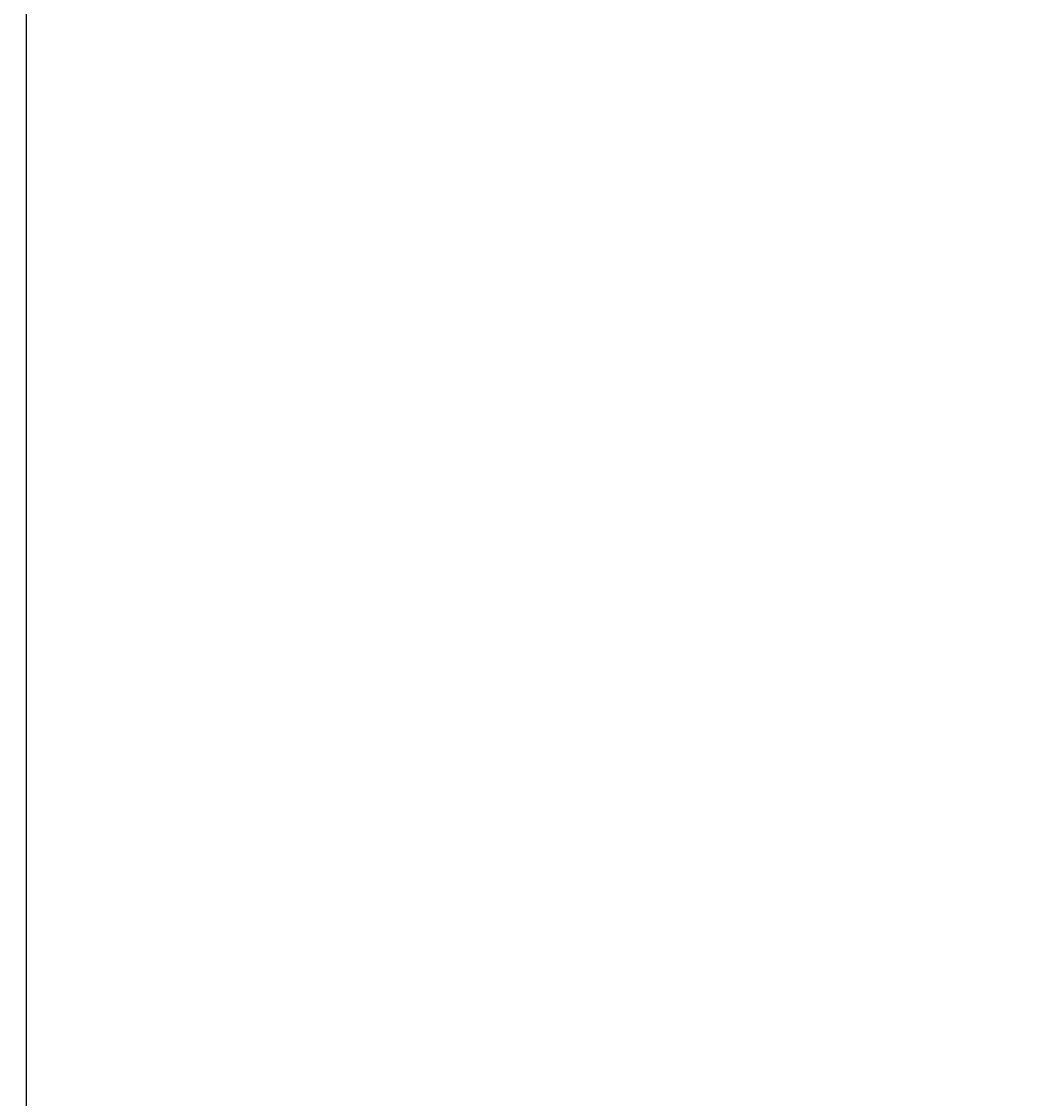
# Model space of a CAD drawing. Units: millimetres. Extents: x 27017497 to 27018854, y 7058029 to 7059154.
# Tile 2 of 91: x 27017497 to 27017560, y 7058133 to 7058200. Entities that reach past the tile are written whole.
import ezdxf

# ---------------------------------------------------------------- set-up
doc = ezdxf.new("R2010")
doc.units = ezdxf.units.MM
doc.layers.add('A-ANNO-DIMS', color=2, linetype='Continuous', lineweight=18)
doc.styles.get("Standard").update_dxf_attribs({"font": 'arial.ttf'})
doc.dimstyles.get("Standard").update_dxf_attribs({"dimtxt": 0.18, "dimasz": 0.18, "dimexe": 0.18, "dimexo": 0.0625, "dimgap": 0.09, "dimtad": 0, "dimtih": 1, "dimtoh": 1, "dimdec": 4, "dimzin": 0, "dimdsep": 46, "dimtxsty": 'Standard', "dimcen": 0.09, "dimadec": 0, "dimazin": 0, "dimtfac": 1, "dimtdec": 4, "dimtofl": 0, "dimtmove": 0, "dimatfit": 3, "dimfxl": 1, "dimtolj": 1, "dimtzin": 0, "dimarcsym": 0})

# ---------------------------------------------------------------- blocks, each defined once
blk = doc.blocks.new('*D48')
at = {"layer": 'A-ANNO-DIMS', "color": 0, "lineweight": -2, "transparency": 16777216}
for p, q in [((27018463.498, 7058622.912), (27017497.536, 7058622.912)), ((27017497.716, 7058622.732), (27017497.716, 7058357.753)), ((27017497.716, 7058092.41), (27017497.716, 7058357.389)), ((27018555.129, 7058092.23), (27017497.536, 7058092.23))]:
    blk.add_line(p, q, dxfattribs=at)
at = {"layer": 'A-ANNO-DIMS', "color": 0, "transparency": 16777216}
for points in [[(27017497.686, 7058622.732), (27017497.746, 7058622.732), (27017497.716, 7058622.912)], [(27017497.686, 7058092.41), (27017497.746, 7058092.41), (27017497.716, 7058092.23)]]:
    blk.add_solid(points, dxfattribs=at)
at = {"layer": 'Defpoints', "color": 0, "transparency": 16777216}
for p in [(27018463.561, 7058622.912), (27017497.716, 7058092.23), (27018555.192, 7058092.23)]:
    blk.add_point(p, dxfattribs=at)
at = {"layer": 'A-ANNO-DIMS', "color": 0, "transparency": 16777216, "insert": (27017497.716, 7058357.571), "char_height": 0.18, "attachment_point": 5}
blk.add_mtext('\\A1;530.7', dxfattribs=at)

msp = doc.modelspace()

# ---------------------------------------------------------------- dimensions: what is measured, and where the dimension line sits
at = {"layer": 'A-ANNO-DIMS'}
dim = msp.add_linear_dim(base=(27017497.716, 7058092.23), p1=(27018463.561, 7058622.912), p2=(27018555.192, 7058092.23), angle=90, dimstyle='Standard', override={"dimdec": 1, "dimlfac": 1, "dimrnd": 0, "dimzin": 0, "dimdsep": 46, "dimlunit": 2}, dxfattribs=at)
dim.commit()
dim.dimension.update_dxf_attribs({"geometry": '*D48', "text_midpoint": (27017497.716, 7058357.571)})

doc.saveas('drawing.dxf')
